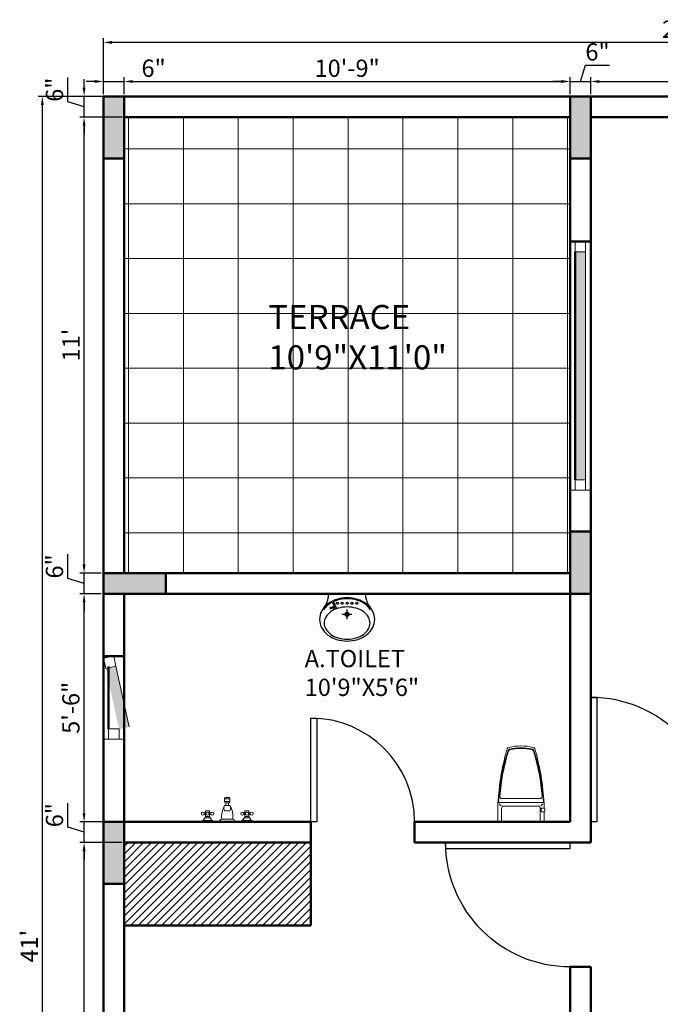
# Model space of a CAD drawing. Units: inches. Extents: x 3064 to 19385, y 846 to 15425.
# Tile 43 of 108: x 5167 to 5352, y 1129 to 1414. Entities that reach past the tile are written whole.
import ezdxf

# ---------------------------------------------------------------- set-up
doc = ezdxf.new("R2010")
doc.units = ezdxf.units.IN
for name, color, linetype, lineweight in [('A-ANNO-DIMS', 2, 'Continuous', 18), ('A-AREA-IDEN', 3, 'Continuous', 18), ('A-COLS', 1, 'Continuous', 35), ('A-DOOR', 3, 'Continuous', 25), ('A-FLOR-FIXT', 9, 'Continuous', 18), ('A-FLOR-PATT', 252, 'Continuous', 13), ('A-FURN-PATT', 252, 'Continuous', 13), ('A-GLAZ', 4, 'Continuous', 18), ('A-WALL', 7, 'Continuous', 50)]:
    doc.layers.add(name, color=color, linetype=linetype, lineweight=lineweight)
doc.layers.add('THIET-BI', color=21, linetype='Continuous')
doc.styles.get("Standard").update_dxf_attribs({"font": 'arial.ttf'})
doc.dimstyles.new('ISO-25', dxfattribs={"dimtxt": 9, "dimasz": 2.5, "dimexe": 1.25, "dimexo": 0.625, "dimtad": 1, "dimdec": 1, "dimlunit": 3, "dimtxsty": 'Standard', "dimcen": 2.5, "dimadec": 0, "dimazin": 0, "dimtfac": 1, "dimtdec": 1, "dimtmove": 0, "dimatfit": 3, "dimfxl": 1, "dimarcsym": 0})

# ---------------------------------------------------------------- blocks, each defined once
blk = doc.blocks.new('*U3')
for p, q in [((0, 0), (0, -6)), ((36, 0), (36, -6))]:
    blk.add_line(p, q)
blk.add_lwpolyline([(0, 0), (0, 36), (1.75, 36), (1.75, 0)], close=True)
blk.add_arc((0, 0), 36, 0, 90)
blk = doc.blocks.new('*U4')
for p, q in [((0, 0), (0, -6)), ((30, 0), (30, -6))]:
    blk.add_line(p, q)
blk.add_lwpolyline([(0, 0), (0, 30), (1.75, 30), (1.75, 0)], close=True)
blk.add_arc((0, 0), 30, 0, 90)
blk = doc.blocks.new('A$C430D11A0')
at = {"layer": 'THIET-BI'}
for p, q in [((90, 445), (90, 485)), ((475, 485), (90, 485)), ((475, 483), (90, 483)), ((475, 445), (475, 485)), ((129, 398), (158, 344)), ((138, 403), (176, 332)), ((282, 226), (282, 325)), ((233, 275), (332, 275))]:
    blk.add_line(p, q, dxfattribs=at)
for points in [[(565, 223, 0.121635), (545, 305, 0.10526), (482, 380, 0.088175), (393, 427, 0.079002), (282, 445, 0.079002), (172, 427, 0.088175), (83, 380, 0.10526), (20, 305, 0.121635), (0, 223, 0.121635), (20, 140, 0.10526), (83, 65, 0.088175), (172, 18, 0.079002), (282, 0, 0.079002), (393, 18, 0.088175), (482, 65, 0.10526), (545, 140, 0.121635)], [(517, 185, 0.134042), (501, 245, 0.106817), (449, 302, 0.082468), (376, 337, 0.070874), (282, 350, 0.070874), (189, 337, 0.082468), (116, 302, 0.106817), (64, 245, 0.134042), (47, 185, 0.134042), (64, 125, 0.106817), (116, 68, 0.082468), (189, 33, 0.070874), (282, 20, 0.070874), (376, 33, 0.082468), (449, 68, 0.106817), (501, 125, 0.134042)]]:
    blk.add_lwpolyline(points, format="xyb", close=True, dxfattribs=at)
for points in [[(523, 322, 0.07708), (476, 372, 0.088175), (390, 418, 0.079002), (282, 435, 0.079002), (175, 418, 0.035427), (138, 403, 0.07708)], [(129, 398, 0.043566), (89, 372, 0.07708), (42, 322, 0.041486)]]:
    blk.add_lwpolyline(points, format="xyb", dxfattribs=at)
for centre, radius in [((182, 388), 10.5), ((232, 388), 10.5), ((282, 388), 10.5), ((332, 388), 10.5), ((382, 388), 10.5), ((282, 275), 20), ((282, 275), 15)]:
    blk.add_circle(centre, radius, dxfattribs=at)
for centre, radius, start, end in [((-104, 469), 195, 320.8253, 352.9557), ((669, 469), 195, 187.0443, 219.1747), ((136, 285), 62.9, 69.643, 123.4774), ((136, 285), 52.9, 55.2455, 123.4774)]:
    blk.add_arc(centre, radius, start, end, dxfattribs=at)
blk = doc.blocks.new('WC-P05')
for p, q in [((-202, 532), (-202, 439)), ((-192, 542), (263, 542)), ((-163, 542), (-163, 401)), ((234, 542), (234, 401)), ((273, 532), (273, 352)), ((-210, 430), (-210, 409)), ((-201, 439), (-180, 439)), ((-171, 430), (-171, 409)), ((-202, 400), (-202, 352)), ((-201, 400), (-180, 400)), ((-192, 342), (263, 342)), ((-167, 379), (-188, 357)), ((-143, 381), (214, 381)), ((237, 379), (258, 357)), ((-159, 303), (229, 303))]:
    blk.add_line(p, q)
blk.add_lwpolyline([(-91, -222, 0.114547), (161, -222, 0.114547)], format="xyb")
for centre, radius, start, end in [((-192, 532), 10, 90, 180), ((263, 532), 10, 0, 90), ((-201, 430), 9, 90, 180), ((-201, 409), 9, 180, 270), ((-180, 430), 9, 0, 90), ((-180, 409), 9, 270, 0), ((2309, 492), 2515, 183.2067, 196.1242), ((-192, 352), 10, 180, 270), ((1906, 447), 2103, 182.8743, 197.6554), ((-143, 401), 20, 180, 270), ((-1836, 447), 2103, 342.3446, 357.1257), ((-2239, 492), 2515, 343.8727, 356.7933), ((214, 401), 20, 270, 0), ((263, 352), 10, 270, 0), ((-159, 280), 22.5, 90, 184.6246), ((1906, 447), 2095, 184.6245, 197.5277), ((-1836, 447), 2095, 342.464, 355.3754), ((229, 280), 22.5, 355.3754, 90), ((-76, -184), 22.5, 197.6554, 257.5059), ((-70, -177), 22.5, 197.5277, 258.1005), ((36, 324), 535, 258.1005, 281.7373), ((140, -177), 22.5, 281.7373, 342.464), ((146, -184), 22.5, 282.4941, 342.3446), ((-86, -200), 22.5, 196.1242, 256.8994), ((35, 318), 536, 257.5059, 282.4941), ((156, -200), 22.5, 283.0378, 343.8727)]:
    blk.add_arc(centre, radius, start, end)
blk = doc.blocks.new('Faucet - Bathroom front')
for p, q in [((-0.5, 4.25), (0.5, 4.25)), ((0.5, 3.75), (-0.5, 3.75)), ((-0.5, 3), (0.5, 3)), ((0.5, 2), (-0.5, 2)), ((-0.25, 3), (-0.25, 3.5)), ((0.25, 3.5), (0.25, 3)), ((-5, 0), (-2.25, 0)), ((-4.5087, 0.25), (-2.7408, 0.25)), ((-4, 1.625), (-4.25, 1.625)), ((-4, 1.375), (-4.25, 1.375)), ((-3.1442, 0.75), (-4.0979, 0.75)), ((-3.25, 1.625), (-3, 1.625)), ((-3.25, 1.375), (-3, 1.375)), ((-1.5, 0), (1.5, 0)), ((-1, 0.5), (1, 0.5)), ((2.25, 0), (5, 0)), ((2.7413, 0.25), (4.5092, 0.25)), ((3.25, 1.625), (3, 1.625)), ((3.25, 1.375), (3, 1.375)), ((4.1058, 0.75), (3.1521, 0.75)), ((4, 1.625), (4.25, 1.625)), ((4, 1.375), (4.25, 1.375))]:
    blk.add_line(p, q)
for points in [[(-0.5, 3.75), (-0.5, 4.25)], [(-0.25, 4.5), (0.25, 4.5)], [(0.5, 4.25), (0.5, 3.75)], [(0.25, 3.5), (-0.25, 3.5)]]:
    blk.add_lwpolyline(points)
for points in [[(-4, 1), (-4, 2), (-3.25, 2), (-3.25, 1)], [(3.25, 1), (3.25, 2), (4, 2), (4, 1)]]:
    blk.add_lwpolyline(points, close=True)
for centre in [(-4.5, 1.5), (-3.625, 1.5), (-2.75, 1.5), (2.75, 1.5), (3.625, 1.5), (4.5, 1.5)]:
    blk.add_circle(centre, 0.2795)
for centre, radius, start, end in [((-0.2575, 4.2575), 0.2426, 88.22243, 181.7776), ((-0.2575, 3.7425), 0.2426, 178.2224, 271.7776), ((0.2575, 4.2575), 0.2426, 358.2224, 91.77757), ((0.2575, 3.7425), 0.2426, 268.2224, 1.777565), ((3, 1), 4.0311, 150.2551, 187.125), ((0.6413, 2.5), 1.246, 156.3417, 203.6583), ((-3, 1), 4.0311, 352.875, 29.74488), ((-0.6413, 2.5), 1.246, 336.3417, 23.65835), ((-5.375, 1.375), 1.4252, 285.2551, 344.7449), ((-1.875, 1.375), 1.4252, 195.2551, 254.7449), ((-0.7962, -0.2038), 0.7327, 106.1502, 163.8498), ((0.7962, -0.2038), 0.7327, 16.1502, 73.84979), ((1.875, 1.375), 1.4252, 285.2551, 344.7449), ((5.375, 1.375), 1.4252, 195.2551, 254.7449)]:
    blk.add_arc(centre, radius, start, end)
blk = doc.blocks.new('*D70')
at = {"layer": 'A-ANNO-DIMS', "color": 0, "lineweight": -2, "transparency": 16777216}
for p, q in [((5196.39, 1176.1), (5184.17, 1176.1)), ((5185.42, 980.6), (5185.42, 1173.6)), ((5196.39, 978.1), (5184.17, 978.1))]:
    blk.add_line(p, q, dxfattribs=at)
at = {"layer": 'A-ANNO-DIMS', "color": 0, "transparency": 16777216}
for points in [[(5185, 1173.6), (5185.83, 1173.6), (5185.42, 1176.1)], [(5185, 980.6), (5185.83, 980.6), (5185.42, 978.1)]]:
    blk.add_solid(points, dxfattribs=at)
at = {"layer": 'Defpoints', "color": 0, "transparency": 16777216}
for p in [(5185.42, 1176.1), (5197.02, 1176.1), (5197.02, 978.1)]:
    blk.add_point(p, dxfattribs=at)
at = {"layer": 'A-ANNO-DIMS', "color": 0, "transparency": 16777216, "insert": (5182.24, 1077.1), "char_height": 5, "attachment_point": 5, "rotation": 90}
blk.add_mtext('16\'-6"', dxfattribs=at)
blk = doc.blocks.new('*D71')
at = {"layer": 'A-ANNO-DIMS', "color": 0, "lineweight": -2, "transparency": 16777216}
for p, q in [((5180.68, 1180.52), (5180.68, 1187.54)), ((5185.42, 1184.6), (5185.42, 1187.1)), ((5185.42, 1179.1), (5180.68, 1180.52)), ((5196.39, 1182.1), (5184.17, 1182.1)), ((5185.42, 1176.1), (5185.42, 1182.1)), ((5185.42, 1176.1), (5185.42, 1182.1)), ((5196.39, 1176.1), (5184.17, 1176.1)), ((5185.42, 1173.6), (5185.42, 1171.1))]:
    blk.add_line(p, q, dxfattribs=at)
at = {"layer": 'A-ANNO-DIMS', "color": 0, "transparency": 16777216}
for points in [[(5185, 1184.6), (5185.83, 1184.6), (5185.42, 1182.1)], [(5185, 1173.6), (5185.83, 1173.6), (5185.42, 1176.1)]]:
    blk.add_solid(points, dxfattribs=at)
at = {"layer": 'Defpoints', "color": 0, "transparency": 16777216}
for p in [(5185.42, 1182.1), (5197.02, 1182.1), (5197.02, 1176.1)]:
    blk.add_point(p, dxfattribs=at)
at = {"layer": 'A-ANNO-DIMS', "color": 0, "transparency": 16777216, "insert": (5177.5, 1184.03), "char_height": 5, "attachment_point": 5, "rotation": 90}
blk.add_mtext('6"', dxfattribs=at)
blk = doc.blocks.new('*D72')
at = {"layer": 'A-ANNO-DIMS', "color": 0, "lineweight": -2, "transparency": 16777216}
for p, q in [((5190.39, 1248.1), (5184.17, 1248.1)), ((5185.42, 1184.6), (5185.42, 1245.6)), ((5196.39, 1182.1), (5184.17, 1182.1))]:
    blk.add_line(p, q, dxfattribs=at)
at = {"layer": 'A-ANNO-DIMS', "color": 0, "transparency": 16777216}
for points in [[(5185, 1245.6), (5185.83, 1245.6), (5185.42, 1248.1)], [(5185, 1184.6), (5185.83, 1184.6), (5185.42, 1182.1)]]:
    blk.add_solid(points, dxfattribs=at)
at = {"layer": 'Defpoints', "color": 0, "transparency": 16777216}
for p in [(5185.42, 1248.1), (5191.02, 1248.1), (5197.02, 1182.1)]:
    blk.add_point(p, dxfattribs=at)
at = {"layer": 'A-ANNO-DIMS', "color": 0, "transparency": 16777216, "insert": (5182.24, 1215.1), "char_height": 5, "attachment_point": 5, "rotation": 90}
blk.add_mtext('5\'-6"', dxfattribs=at)
blk = doc.blocks.new('*D73')
at = {"layer": 'A-ANNO-DIMS', "color": 0, "lineweight": -2, "transparency": 16777216}
for p, q in [((5180.68, 1252.52), (5180.68, 1259.54)), ((5185.42, 1256.6), (5185.42, 1259.1)), ((5190.39, 1254.1), (5184.17, 1254.1)), ((5185.42, 1248.1), (5185.42, 1254.1)), ((5185.42, 1248.1), (5185.42, 1254.1)), ((5185.42, 1251.1), (5180.68, 1252.52)), ((5190.39, 1248.1), (5184.17, 1248.1)), ((5185.42, 1245.6), (5185.42, 1243.1))]:
    blk.add_line(p, q, dxfattribs=at)
at = {"layer": 'A-ANNO-DIMS', "color": 0, "transparency": 16777216}
for points in [[(5185, 1256.6), (5185.83, 1256.6), (5185.42, 1254.1)], [(5185, 1245.6), (5185.83, 1245.6), (5185.42, 1248.1)]]:
    blk.add_solid(points, dxfattribs=at)
at = {"layer": 'Defpoints', "color": 0, "transparency": 16777216}
for p in [(5185.42, 1254.1), (5191.02, 1254.1), (5191.02, 1248.1)]:
    blk.add_point(p, dxfattribs=at)
at = {"layer": 'A-ANNO-DIMS', "color": 0, "transparency": 16777216, "insert": (5177.5, 1256.03), "char_height": 5, "attachment_point": 5, "rotation": 90}
blk.add_mtext('6"', dxfattribs=at)
blk = doc.blocks.new('*D74')
at = {"layer": 'A-ANNO-DIMS', "color": 0, "lineweight": -2, "transparency": 16777216}
for p, q in [((5196.39, 1386.1), (5184.17, 1386.1)), ((5185.42, 1256.6), (5185.42, 1383.6)), ((5190.39, 1254.1), (5184.17, 1254.1))]:
    blk.add_line(p, q, dxfattribs=at)
at = {"layer": 'A-ANNO-DIMS', "color": 0, "transparency": 16777216}
for points in [[(5185, 1383.6), (5185.83, 1383.6), (5185.42, 1386.1)], [(5185, 1256.6), (5185.83, 1256.6), (5185.42, 1254.1)]]:
    blk.add_solid(points, dxfattribs=at)
at = {"layer": 'Defpoints', "color": 0, "transparency": 16777216}
for p in [(5185.42, 1386.1), (5197.02, 1386.1), (5191.02, 1254.1)]:
    blk.add_point(p, dxfattribs=at)
at = {"layer": 'A-ANNO-DIMS', "color": 0, "transparency": 16777216, "insert": (5182.28, 1320.1), "char_height": 5, "attachment_point": 5, "rotation": 90}
blk.add_mtext("11'", dxfattribs=at)
blk = doc.blocks.new('*D75')
at = {"layer": 'A-ANNO-DIMS', "color": 0, "lineweight": -2, "transparency": 16777216}
for p, q in [((5180.68, 1390.52), (5180.68, 1397.54)), ((5185.42, 1394.6), (5185.42, 1397.1)), ((5196.39, 1392.1), (5184.17, 1392.1)), ((5185.42, 1386.1), (5185.42, 1392.1)), ((5185.42, 1386.1), (5185.42, 1392.1)), ((5185.42, 1389.1), (5180.68, 1390.52)), ((5196.39, 1386.1), (5184.17, 1386.1)), ((5185.42, 1383.6), (5185.42, 1381.1))]:
    blk.add_line(p, q, dxfattribs=at)
at = {"layer": 'A-ANNO-DIMS', "color": 0, "transparency": 16777216}
for points in [[(5185, 1394.6), (5185.83, 1394.6), (5185.42, 1392.1)], [(5185, 1383.6), (5185.83, 1383.6), (5185.42, 1386.1)]]:
    blk.add_solid(points, dxfattribs=at)
at = {"layer": 'Defpoints', "color": 0, "transparency": 16777216}
for p in [(5185.42, 1392.1), (5197.02, 1392.1), (5197.02, 1386.1)]:
    blk.add_point(p, dxfattribs=at)
at = {"layer": 'A-ANNO-DIMS', "color": 0, "transparency": 16777216, "insert": (5177.5, 1394.03), "char_height": 5, "attachment_point": 5, "rotation": 90}
blk.add_mtext('6"', dxfattribs=at)
blk = doc.blocks.new('*D76')
at = {"layer": 'A-ANNO-DIMS', "color": 0, "lineweight": -2, "transparency": 16777216}
for p, q in [((5190.39, 1392.1), (5172.09, 1392.1)), ((5173.34, 902.6), (5173.34, 1389.6)), ((5190.39, 900.1), (5172.09, 900.1))]:
    blk.add_line(p, q, dxfattribs=at)
at = {"layer": 'A-ANNO-DIMS', "color": 0, "transparency": 16777216}
for points in [[(5172.92, 1389.6), (5173.75, 1389.6), (5173.34, 1392.1)], [(5172.92, 902.6), (5173.75, 902.6), (5173.34, 900.1)]]:
    blk.add_solid(points, dxfattribs=at)
at = {"layer": 'Defpoints', "color": 0, "transparency": 16777216}
for p in [(5173.34, 1392.1), (5191.02, 1392.1), (5191.02, 900.1)]:
    blk.add_point(p, dxfattribs=at)
at = {"layer": 'A-ANNO-DIMS', "color": 0, "transparency": 16777216, "insert": (5170.2, 1146.1), "char_height": 5, "attachment_point": 5, "rotation": 90}
blk.add_mtext("41'", dxfattribs=at)
blk = doc.blocks.new('*D89')
at = {"layer": 'A-ANNO-DIMS', "color": 0, "lineweight": -2, "transparency": 16777216}
for p, q in [((5191.02, 1392.72), (5191.02, 1397.66)), ((5197.02, 1392.72), (5197.02, 1397.66)), ((5188.52, 1396.41), (5186.02, 1396.41)), ((5191.02, 1396.41), (5197.02, 1396.41)), ((5199.52, 1396.41), (5209.04, 1396.41))]:
    blk.add_line(p, q, dxfattribs=at)
at = {"layer": 'A-ANNO-DIMS', "color": 0, "transparency": 16777216}
for points in [[(5188.52, 1396.83), (5188.52, 1395.99), (5191.02, 1396.41)], [(5199.52, 1396.83), (5199.52, 1395.99), (5197.02, 1396.41)]]:
    blk.add_solid(points, dxfattribs=at)
at = {"layer": 'Defpoints', "color": 0, "transparency": 16777216}
for p in [(5197.02, 1396.41), (5191.02, 1392.1), (5197.02, 1392.1)]:
    blk.add_point(p, dxfattribs=at)
at = {"layer": 'A-ANNO-DIMS', "color": 0, "transparency": 16777216, "insert": (5205.53, 1399.59), "char_height": 5, "attachment_point": 5}
blk.add_mtext('6"', dxfattribs=at)
blk = doc.blocks.new('*D90')
at = {"layer": 'A-ANNO-DIMS', "color": 0, "lineweight": -2, "transparency": 16777216}
for p, q in [((5197.02, 1392.72), (5197.02, 1397.66)), ((5326.02, 1392.72), (5326.02, 1397.66)), ((5199.52, 1396.41), (5323.52, 1396.41))]:
    blk.add_line(p, q, dxfattribs=at)
at = {"layer": 'A-ANNO-DIMS', "color": 0, "transparency": 16777216}
for points in [[(5199.52, 1396.83), (5199.52, 1395.99), (5197.02, 1396.41)], [(5323.52, 1396.83), (5323.52, 1395.99), (5326.02, 1396.41)]]:
    blk.add_solid(points, dxfattribs=at)
at = {"layer": 'Defpoints', "color": 0, "transparency": 16777216}
for p in [(5326.02, 1396.41), (5197.02, 1392.1), (5326.02, 1392.1)]:
    blk.add_point(p, dxfattribs=at)
at = {"layer": 'A-ANNO-DIMS', "color": 0, "transparency": 16777216, "insert": (5261.52, 1399.59), "char_height": 5, "attachment_point": 5}
blk.add_mtext('10\'-9"', dxfattribs=at)
blk = doc.blocks.new('*D91')
at = {"layer": 'A-ANNO-DIMS', "color": 0, "lineweight": -2, "transparency": 16777216}
for p, q in [((5329.02, 1396.41), (5330.44, 1401.15)), ((5330.44, 1401.15), (5337.46, 1401.15)), ((5326.02, 1392.72), (5326.02, 1397.66)), ((5332.02, 1392.72), (5332.02, 1397.66)), ((5323.52, 1396.41), (5321.02, 1396.41)), ((5326.02, 1396.41), (5332.02, 1396.41)), ((5326.02, 1396.41), (5332.02, 1396.41)), ((5334.52, 1396.41), (5337.02, 1396.41))]:
    blk.add_line(p, q, dxfattribs=at)
at = {"layer": 'A-ANNO-DIMS', "color": 0, "transparency": 16777216}
for points in [[(5323.52, 1396.83), (5323.52, 1395.99), (5326.02, 1396.41)], [(5334.52, 1396.83), (5334.52, 1395.99), (5332.02, 1396.41)]]:
    blk.add_solid(points, dxfattribs=at)
at = {"layer": 'Defpoints', "color": 0, "transparency": 16777216}
for p in [(5332.02, 1396.41), (5326.02, 1392.1), (5332.02, 1392.1)]:
    blk.add_point(p, dxfattribs=at)
at = {"layer": 'A-ANNO-DIMS', "color": 0, "transparency": 16777216, "insert": (5333.95, 1404.33), "char_height": 5, "attachment_point": 5}
blk.add_mtext('6"', dxfattribs=at)
blk = doc.blocks.new('*D92')
at = {"layer": 'A-ANNO-DIMS', "color": 0, "lineweight": -2, "transparency": 16777216}
for p, q in [((5332.02, 1392.72), (5332.02, 1397.66)), ((5527.02, 1392.72), (5527.02, 1397.66)), ((5334.52, 1396.41), (5524.52, 1396.41))]:
    blk.add_line(p, q, dxfattribs=at)
at = {"layer": 'A-ANNO-DIMS', "color": 0, "transparency": 16777216}
for points in [[(5334.52, 1396.83), (5334.52, 1395.99), (5332.02, 1396.41)], [(5524.52, 1396.83), (5524.52, 1395.99), (5527.02, 1396.41)]]:
    blk.add_solid(points, dxfattribs=at)
at = {"layer": 'Defpoints', "color": 0, "transparency": 16777216}
for p in [(5527.02, 1396.41), (5332.02, 1392.1), (5527.02, 1392.1)]:
    blk.add_point(p, dxfattribs=at)
at = {"layer": 'A-ANNO-DIMS', "color": 0, "transparency": 16777216, "insert": (5429.52, 1399.59), "char_height": 5, "attachment_point": 5}
blk.add_mtext('16\'-3"', dxfattribs=at)
blk = doc.blocks.new('*D94')
at = {"layer": 'A-ANNO-DIMS', "color": 0, "lineweight": -2, "transparency": 16777216}
for p, q in [((5191.02, 1392.72), (5191.02, 1408.96)), ((5533.02, 1392.72), (5533.02, 1408.96)), ((5530.52, 1407.71), (5193.52, 1407.71))]:
    blk.add_line(p, q, dxfattribs=at)
at = {"layer": 'A-ANNO-DIMS', "color": 0, "transparency": 16777216}
for points in [[(5193.52, 1408.12), (5193.52, 1407.29), (5191.02, 1407.71)], [(5530.52, 1408.12), (5530.52, 1407.29), (5533.02, 1407.71)]]:
    blk.add_solid(points, dxfattribs=at)
at = {"layer": 'Defpoints', "color": 0, "transparency": 16777216}
for p in [(5191.02, 1407.71), (5191.02, 1392.1), (5533.02, 1392.1)]:
    blk.add_point(p, dxfattribs=at)
at = {"layer": 'A-ANNO-DIMS', "color": 0, "transparency": 16777216, "insert": (5362.02, 1410.88), "char_height": 5, "attachment_point": 5}
blk.add_mtext('28\'-6"', dxfattribs=at)
blk = doc.blocks.new('WIN-600')
h = blk.add_hatch(color=256)
h.dxf.hatch_style = 1
h.paths.add_polyline_path([(3, 18), (0, 18), (0, 0), (3, 0)])
blk.add_line((3, 18), (3, 0))
blk.add_lwpolyline([(3, 18), (0, 18), (0, 21), (3, 21)], close=True)
blk = doc.blocks.new('WIN-1900')
blk.add_line((3, 0), (3, 66))
blk.add_lwpolyline([(3, 66), (0, 66), (0, 69), (3, 69)], close=True)

msp = doc.modelspace()

# ---------------------------------------------------------------- hatches: boundary and pattern name
at = {"layer": 'A-COLS'}
h = msp.add_hatch(color=256, dxfattribs=at)
h.dxf.hatch_style = 1
h.paths.add_polyline_path([(5197.02, 1374.1), (5197.02, 1392.1), (5191.02, 1392.1), (5191.02, 1374.1)])
h = msp.add_hatch(color=256, dxfattribs=at)
h.dxf.hatch_style = 1
h.paths.add_polyline_path([(5332.02, 1374.1), (5332.02, 1392.1), (5326.02, 1392.1), (5326.02, 1374.1)])
h = msp.add_hatch(color=256, dxfattribs=at)
h.dxf.hatch_style = 1
h.paths.add_polyline_path([(5332.02, 1248.1), (5332.02, 1266.1), (5326.02, 1266.1), (5326.02, 1248.1)])
h = msp.add_hatch(color=256, dxfattribs=at)
h.dxf.hatch_style = 1
h.paths.add_polyline_path([(5209.02, 1254.1), (5191.02, 1254.1), (5191.02, 1248.1), (5209.02, 1248.1)])
h = msp.add_hatch(color=256, dxfattribs=at)
h.dxf.hatch_style = 1
h.paths.add_polyline_path([(5197.02, 1164.1), (5197.02, 1182.1), (5191.02, 1182.1), (5191.02, 1164.1)])
at = {"layer": 'A-FLOR-PATT'}
h = msp.add_hatch(dxfattribs=at)
h.set_pattern_fill('ANSI37', color=256, scale=5, angle=45)
h.set_pattern_definition([(90, (848.524, -4.244), (-15.875, 0), []), (180, (848.524, -4.244), (-2e-15, -15.875), [])])
h.paths.add_polyline_path([(5197.02, 1386.1), (5197.02, 1374.1), (5197.02, 1254.1), (5326.02, 1254.1), (5326.02, 1266.1), (5326.02, 1386.1)])
at = {"layer": 'A-FURN-PATT'}
h = msp.add_hatch(dxfattribs=at)
h.set_pattern_fill('ANSI31', color=256, scale=0.5)
h.set_pattern_definition([(45, (848.524, -10.2436), (-1.122532, 1.122532), [])])
h.paths.add_polyline_path([(5251.02, 1176.1), (5197.02, 1176.1), (5197.02, 1158.1), (5197.02, 1152.1), (5251.02, 1152.1)])
at = {"layer": 'A-GLAZ'}
h = msp.add_hatch(color=256, dxfattribs=at)
h.dxf.hatch_style = 1
h.paths.add_polyline_path([(5327.52, 1281.1), (5330.52, 1281.1), (5330.52, 1347.1), (5327.52, 1347.1)])

# ---------------------------------------------------------------- linework, layer by layer
for p, q in [((5332.02, 1278.1), (5326.02, 1278.1)), ((5191.02, 1206.03), (5197.02, 1206.03))]:
    msp.add_line(p, q, dxfattribs=at)
for points in [[(5330.52, 1278.1), (5327.52, 1278.1), (5327.52, 1281.1), (5330.52, 1281.1)], [(5195.52, 1206.03), (5192.52, 1206.03), (5192.52, 1209.03), (5195.52, 1209.03)]]:
    msp.add_lwpolyline(points, close=True, dxfattribs=at)
at = {"layer": 'A-WALL'}
for p, q in [((5533.02, 1392.1), (5191.02, 1392.1)), ((5191.02, 1392.1), (5191.02, 972.1)), ((5326.02, 1386.1), (5197.02, 1386.1)), ((5197.02, 1386.1), (5197.02, 1254.1)), ((5326.02, 1386.1), (5326.02, 1254.1)), ((5527.02, 1386.1), (5332.02, 1386.1)), ((5332.02, 1386.1), (5332.02, 1176.1)), ((5326.02, 1350.1), (5332.02, 1350.1)), ((5327.52, 1347.1), (5327.52, 1281.1)), ((5197.02, 1254.1), (5326.02, 1254.1)), ((5197.02, 1248.1), (5197.02, 1182.1)), ((5197.02, 1248.1), (5326.02, 1248.1)), ((5332.02, 1248.1), (5326.02, 1248.1)), ((5326.02, 1248.1), (5326.02, 1182.1)), ((5191.02, 1230.03), (5197.02, 1230.03)), ((5192.52, 1227.03), (5192.52, 1209.03)), ((5197.02, 1182.1), (5251.02, 1182.1)), ((5251.02, 1182.1), (5251.02, 1152.1)), ((5281.02, 1182.1), (5326.02, 1182.1)), ((5281.02, 1182.1), (5281.02, 1176.1)), ((5197.02, 1176.1), (5197.02, 978.1)), ((5197.02, 1176.1), (5251.02, 1176.1)), ((5281.02, 1176.1), (5332.02, 1176.1)), ((5197.02, 1152.1), (5251.02, 1152.1)), ((5326.02, 1140.1), (5326.02, 978.1)), ((5326.02, 1140.1), (5332.02, 1140.1)), ((5332.02, 1140.1), (5332.02, 972.1))]:
    msp.add_line(p, q, dxfattribs=at)
for points in [[(5197.02, 1374.1), (5197.02, 1392.1), (5191.02, 1392.1), (5191.02, 1374.1)], [(5332.02, 1374.1), (5332.02, 1392.1), (5326.02, 1392.1), (5326.02, 1374.1)], [(5332.02, 1248.1), (5332.02, 1266.1), (5326.02, 1266.1), (5326.02, 1248.1)], [(5209.02, 1254.1), (5191.02, 1254.1), (5191.02, 1248.1), (5209.02, 1248.1)], [(5197.02, 1164.1), (5197.02, 1182.1), (5191.02, 1182.1), (5191.02, 1164.1)]]:
    msp.add_lwpolyline(points, close=True, dxfattribs=at)

# ---------------------------------------------------------------- block references
at = {"layer": 'A-DOOR'}
for name, p in [('*U3', (5332.02, 1182.1)), ('*U4', (5251.02, 1182.1))]:
    msp.add_blockref(name, p, dxfattribs=at)
at = {"layer": 'A-DOOR', "xscale": -1, "rotation": 90}
msp.add_blockref('*U3', (5326.02, 1176.1), dxfattribs=at)
at = {"layer": 'A-FLOR-FIXT'}
for name, p, xscale, yscale, zscale in [('A$C430D11A0', (5253.54, 1234.41), 0.0282220760332506, 0.0282220760332506, 0.0282220760332506), ('Faucet - Bathroom front', (5226.83, 1182.1), 1.573166238287219, 1.573166238287219, 1.573166238287219)]:
    msp.add_blockref(name, p, dxfattribs=dict(at, xscale=xscale, yscale=yscale, zscale=zscale))
at = {"layer": 'A-FLOR-FIXT', "xscale": 0.0282220760332506, "yscale": 0.0282220760332506, "zscale": 0.0282220760332506, "rotation": 180}
msp.add_blockref('WC-P05', (5312.8, 1197.38), dxfattribs=at)
at = {"layer": 'A-GLAZ'}
msp.add_blockref('WIN-1900', (5327.52, 1281.1), dxfattribs=at)
at = {"layer": 'A-GLAZ', "rotation": 12.21571913413454}
msp.add_blockref('WIN-600', (5195.52, 1208.93), dxfattribs=at)

# ---------------------------------------------------------------- texts
at = {"layer": 'A-AREA-IDEN', "attachment_point": 1}
for s, insert, char_height in [('TERRACE\\P10\'9"X11\'0"', (5238.74, 1331.72), 7), ('A.TOILET\\P10\'9"X5\'6"', (5249.24, 1231.86), 5)]:
    msp.add_mtext_dynamic_manual_height_columns(s, width=67.5924, gutter_width=12.5, heights=[0], dxfattribs=dict(at, insert=insert, char_height=char_height))

# ---------------------------------------------------------------- dimensions: what is measured, and where the dimension line sits
at = {"layer": 'A-ANNO-DIMS'}
for base, p1, p2, override, picture, middle in [((5191.02, 1407.71), (5533.02, 1392.1), (5191.02, 1392.1), {"dimtxt": 5, "dimclrd": 0, "dimclre": 0, "dimclrt": 0}, '*D94', (5362.02, 1410.88)), ((5332.02, 1396.41), (5326.02, 1392.1), (5332.02, 1392.1), {"dimtxt": 5, "dimclrd": 0, "dimclre": 0, "dimclrt": 0, "dimtmove": 1}, '*D91', (5331.06, 1404.33)), ((5197.02, 1396.41), (5191.02, 1392.1), (5197.02, 1392.1), {"dimtxt": 5, "dimclrd": 0, "dimclre": 0, "dimclrt": 0}, '*D89', (5205.53, 1399.59)), ((5326.02, 1396.41), (5197.02, 1392.1), (5326.02, 1392.1), {"dimtxt": 5, "dimclrd": 0, "dimclre": 0, "dimclrt": 0, "dimtmove": 1}, '*D90', (5261.52, 1399.59)), ((5527.02, 1396.41), (5332.02, 1392.1), (5527.02, 1392.1), {"dimtxt": 5, "dimclrd": 0, "dimclre": 0, "dimclrt": 0, "dimtmove": 1}, '*D92', (5429.52, 1399.59))]:
    dim = msp.add_linear_dim(base=base, p1=p1, p2=p2, dimstyle='ISO-25', override=override, dxfattribs=at)
    dim.commit()
    dim.dimension.update_dxf_attribs({"geometry": picture, "text_midpoint": middle})
for base, p1, p2, override, picture, middle in [((5185.42, 1392.1), (5197.02, 1386.1), (5197.02, 1392.1), {"dimtxt": 5, "dimclrd": 0, "dimclre": 0, "dimclrt": 0, "dimtmove": 1}, '*D75', (5177.5, 1391.14)), ((5173.34, 1392.1), (5191.02, 900.1), (5191.02, 1392.1), {"dimtxt": 5, "dimclrd": 0, "dimclre": 0, "dimclrt": 0}, '*D76', (5170.2, 1146.1)), ((5185.42, 1386.1), (5191.02, 1254.1), (5197.02, 1386.1), {"dimtxt": 5, "dimclrd": 0, "dimclre": 0, "dimclrt": 0, "dimtmove": 1}, '*D74', (5182.28, 1320.1)), ((5185.42, 1254.1), (5191.02, 1248.1), (5191.02, 1254.1), {"dimtxt": 5, "dimclrd": 0, "dimclre": 0, "dimclrt": 0, "dimtmove": 1}, '*D73', (5177.5, 1253.14)), ((5185.42, 1248.1), (5197.02, 1182.1), (5191.02, 1248.1), {"dimtxt": 5, "dimclrd": 0, "dimclre": 0, "dimclrt": 0, "dimtmove": 1}, '*D72', (5182.24, 1215.1)), ((5185.42, 1182.1), (5197.02, 1176.1), (5197.02, 1182.1), {"dimtxt": 5, "dimclrd": 0, "dimclre": 0, "dimclrt": 0, "dimtmove": 1}, '*D71', (5177.5, 1181.14)), ((5185.42, 1176.1), (5197.02, 978.1), (5197.02, 1176.1), {"dimtxt": 5, "dimclrd": 0, "dimclre": 0, "dimclrt": 0, "dimtmove": 1}, '*D70', (5182.24, 1077.1))]:
    dim = msp.add_linear_dim(base=base, p1=p1, p2=p2, angle=90, dimstyle='ISO-25', override=override, dxfattribs=at)
    dim.commit()
    dim.dimension.update_dxf_attribs({"geometry": picture, "text_midpoint": middle})

doc.saveas('drawing.dxf')
